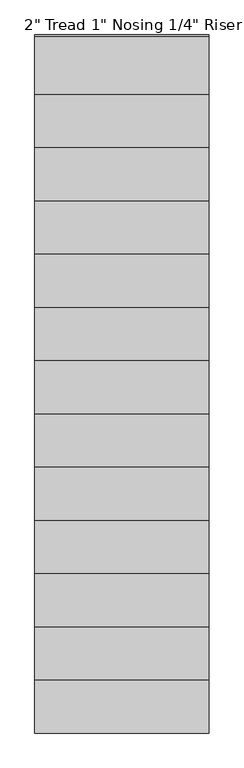
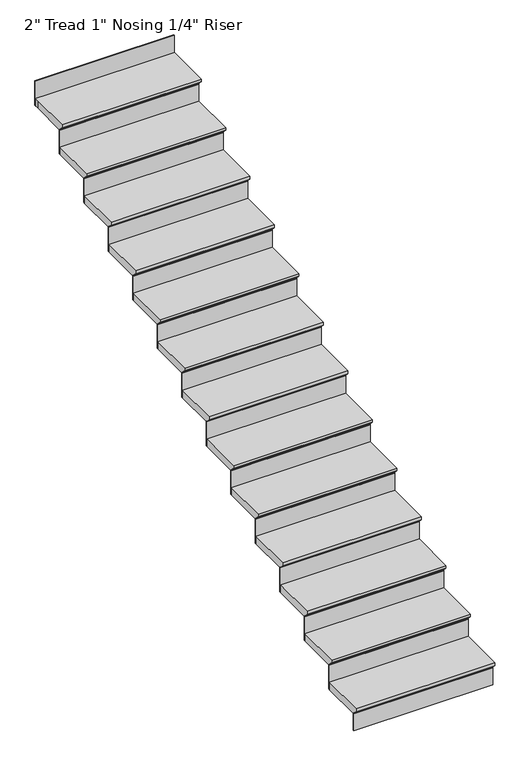
"""IFC4 building model written with IfcOpenShell, lengths in millimetres: stair flight geometry."""

from ifc_helpers import new_model, si_unit, origin, place, context, project, spatial, faceted_brep, source, transform, mapped, element, save


def stair_flight_ca28c9d9(model_context):
    return source(origin(), model_context, "Body", "Brep", [
        faceted_brep([(-2703.0415084, -23154.3851539, 34528.9005799), (-2703.0415084, -23154.3851539, 34547.9505799), (-3617.4415084, -23154.3851539, 34547.9505799), (-3617.4415084, -23154.3851539, 34528.9005799), (-2703.0415084, -23128.9851539, 34503.5005799), (-3617.4415084, -23128.9851539, 34503.5005799), (-2703.0415084, -22849.5851539, 34547.9505799), (-3617.4415084, -22849.5851539, 34547.9505799), (-3617.4415084, -23128.9851539, 34497.1505799), (-3617.4415084, -22849.5851539, 34497.1505799), (-2703.0415084, -22849.5851539, 34497.1505799), (-2703.0415084, -23128.9851539, 34497.1505799)], [[[0, 1, 2, 3]], [[4, 0, 3, 5]], [[2, 1, 6, 7]], [[8, 9, 10, 11]], [[2, 7, 9, 8, 5, 3]], [[8, 11, 4, 5]], [[6, 1, 0, 4, 11, 10]], [[7, 6, 10, 9]]]),
        faceted_brep([(-2703.0415084, -23128.9851539, 34497.1505799), (-2703.0415084, -23128.9851539, 34378.6172466), (-2703.0415084, -23122.6351539, 34378.6172466), (-2703.0415084, -23122.6351539, 34497.1505799), (-3617.4415084, -23128.9851539, 34497.1505799), (-3617.4415084, -23122.6351539, 34497.1505799), (-3617.4415084, -23122.6351539, 34378.6172466), (-3617.4415084, -23128.9851539, 34378.6172466)], [[[0, 1, 2, 3]], [[4, 5, 6, 7]], [[1, 0, 4, 7]], [[2, 1, 7, 6]], [[3, 2, 6, 5]], [[0, 3, 5, 4]]]),
        faceted_brep([(-2703.0415084, -22849.5851539, 34666.4839133), (-2703.0415084, -22849.5851539, 34497.1505799), (-2703.0415084, -22843.2351539, 34497.1505799), (-2703.0415084, -22843.2351539, 34666.4839133), (-3617.4415084, -22849.5851539, 34666.4839133), (-3617.4415084, -22843.2351539, 34666.4839133), (-3617.4415084, -22843.2351539, 34497.1505799), (-3617.4415084, -22849.5851539, 34497.1505799)], [[[0, 1, 2, 3]], [[4, 5, 6, 7]], [[1, 0, 4, 7]], [[2, 1, 7, 6]], [[3, 2, 6, 5]], [[0, 3, 5, 4]]]),
        faceted_brep([(-3617.4415084, -22874.9851539, 34717.2839133), (-2703.0415084, -22874.9851539, 34717.2839133), (-2703.0415084, -22570.1851539, 34717.2839133), (-3617.4415084, -22570.1851539, 34717.2839133), (-3617.4415084, -22849.5851539, 34666.4839133), (-3617.4415084, -22570.1851539, 34666.4839133), (-2703.0415084, -22570.1851539, 34666.4839133), (-2703.0415084, -22849.5851539, 34666.4839133), (-3617.4415084, -22849.5851539, 34672.8339133), (-3617.4415084, -22874.9851539, 34698.2339133), (-2703.0415084, -22849.5851539, 34672.8339133), (-2703.0415084, -22874.9851539, 34698.2339133)], [[[0, 1, 2, 3]], [[4, 5, 6, 7]], [[0, 3, 5, 4, 8, 9]], [[4, 7, 10, 8]], [[2, 1, 11, 10, 7, 6]], [[3, 2, 6, 5]], [[11, 1, 0, 9]], [[10, 11, 9, 8]]]),
        faceted_brep([(-2703.0415084, -22570.1851539, 34835.8172466), (-2703.0415084, -22570.1851539, 34666.4839133), (-2703.0415084, -22563.8351539, 34666.4839133), (-2703.0415084, -22563.8351539, 34835.8172466), (-3617.4415084, -22570.1851539, 34835.8172466), (-3617.4415084, -22563.8351539, 34835.8172466), (-3617.4415084, -22563.8351539, 34666.4839133), (-3617.4415084, -22570.1851539, 34666.4839133)], [[[0, 1, 2, 3]], [[4, 5, 6, 7]], [[1, 0, 4, 7]], [[2, 1, 7, 6]], [[3, 2, 6, 5]], [[0, 3, 5, 4]]]),
        faceted_brep([(-3617.4415084, -22595.5851539, 34886.6172466), (-2703.0415084, -22595.5851539, 34886.6172466), (-2703.0415084, -22290.7851539, 34886.6172466), (-3617.4415084, -22290.7851539, 34886.6172466), (-3617.4415084, -22570.1851539, 34835.8172466), (-3617.4415084, -22290.7851539, 34835.8172466), (-2703.0415084, -22290.7851539, 34835.8172466), (-2703.0415084, -22570.1851539, 34835.8172466), (-3617.4415084, -22570.1851539, 34842.1672466), (-3617.4415084, -22595.5851539, 34867.5672466), (-2703.0415084, -22570.1851539, 34842.1672466), (-2703.0415084, -22595.5851539, 34867.5672466)], [[[0, 1, 2, 3]], [[4, 5, 6, 7]], [[0, 3, 5, 4, 8, 9]], [[4, 7, 10, 8]], [[2, 1, 11, 10, 7, 6]], [[3, 2, 6, 5]], [[11, 1, 0, 9]], [[10, 11, 9, 8]]]),
        faceted_brep([(-2703.0415084, -22290.7851539, 35005.1505799), (-2703.0415084, -22290.7851539, 34835.8172466), (-2703.0415084, -22284.4351539, 34835.8172466), (-2703.0415084, -22284.4351539, 35005.1505799), (-3617.4415084, -22290.7851539, 35005.1505799), (-3617.4415084, -22284.4351539, 35005.1505799), (-3617.4415084, -22284.4351539, 34835.8172466), (-3617.4415084, -22290.7851539, 34835.8172466)], [[[0, 1, 2, 3]], [[4, 5, 6, 7]], [[1, 0, 4, 7]], [[2, 1, 7, 6]], [[3, 2, 6, 5]], [[0, 3, 5, 4]]]),
        faceted_brep([(-3617.4415084, -22316.1851539, 35055.9505799), (-2703.0415084, -22316.1851539, 35055.9505799), (-2703.0415084, -22011.3851539, 35055.9505799), (-3617.4415084, -22011.3851539, 35055.9505799), (-3617.4415084, -22290.7851539, 35005.1505799), (-3617.4415084, -22011.3851539, 35005.1505799), (-2703.0415084, -22011.3851539, 35005.1505799), (-2703.0415084, -22290.7851539, 35005.1505799), (-3617.4415084, -22290.7851539, 35011.5005799), (-3617.4415084, -22316.1851539, 35036.9005799), (-2703.0415084, -22290.7851539, 35011.5005799), (-2703.0415084, -22316.1851539, 35036.9005799)], [[[0, 1, 2, 3]], [[4, 5, 6, 7]], [[0, 3, 5, 4, 8, 9]], [[4, 7, 10, 8]], [[2, 1, 11, 10, 7, 6]], [[3, 2, 6, 5]], [[11, 1, 0, 9]], [[10, 11, 9, 8]]]),
        faceted_brep([(-2703.0415084, -22011.3851539, 35174.4839133), (-2703.0415084, -22011.3851539, 35005.1505799), (-2703.0415084, -22005.0351539, 35005.1505799), (-2703.0415084, -22005.0351539, 35174.4839133), (-3617.4415084, -22011.3851539, 35174.4839133), (-3617.4415084, -22005.0351539, 35174.4839133), (-3617.4415084, -22005.0351539, 35005.1505799), (-3617.4415084, -22011.3851539, 35005.1505799)], [[[0, 1, 2, 3]], [[4, 5, 6, 7]], [[1, 0, 4, 7]], [[2, 1, 7, 6]], [[3, 2, 6, 5]], [[0, 3, 5, 4]]]),
        faceted_brep([(-3617.4415084, -22036.7851539, 35225.2839133), (-2703.0415084, -22036.7851539, 35225.2839133), (-2703.0415084, -21731.9851539, 35225.2839133), (-3617.4415084, -21731.9851539, 35225.2839133), (-3617.4415084, -22011.3851539, 35174.4839133), (-3617.4415084, -21731.9851539, 35174.4839133), (-2703.0415084, -21731.9851539, 35174.4839133), (-2703.0415084, -22011.3851539, 35174.4839133), (-3617.4415084, -22011.3851539, 35180.8339133), (-3617.4415084, -22036.7851539, 35206.2339133), (-2703.0415084, -22011.3851539, 35180.8339133), (-2703.0415084, -22036.7851539, 35206.2339133)], [[[0, 1, 2, 3]], [[4, 5, 6, 7]], [[0, 3, 5, 4, 8, 9]], [[4, 7, 10, 8]], [[2, 1, 11, 10, 7, 6]], [[3, 2, 6, 5]], [[11, 1, 0, 9]], [[10, 11, 9, 8]]]),
        faceted_brep([(-2703.0415084, -21731.9851539, 35343.8172466), (-2703.0415084, -21731.9851539, 35174.4839133), (-2703.0415084, -21725.6351539, 35174.4839133), (-2703.0415084, -21725.6351539, 35343.8172466), (-3617.4415084, -21731.9851539, 35343.8172466), (-3617.4415084, -21725.6351539, 35343.8172466), (-3617.4415084, -21725.6351539, 35174.4839133), (-3617.4415084, -21731.9851539, 35174.4839133)], [[[0, 1, 2, 3]], [[4, 5, 6, 7]], [[1, 0, 4, 7]], [[2, 1, 7, 6]], [[3, 2, 6, 5]], [[0, 3, 5, 4]]]),
        faceted_brep([(-3617.4415084, -21757.3851539, 35394.6172466), (-2703.0415084, -21757.3851539, 35394.6172466), (-2703.0415084, -21452.5851539, 35394.6172466), (-3617.4415084, -21452.5851539, 35394.6172466), (-3617.4415084, -21731.9851539, 35343.8172466), (-3617.4415084, -21452.5851539, 35343.8172466), (-2703.0415084, -21452.5851539, 35343.8172466), (-2703.0415084, -21731.9851539, 35343.8172466), (-3617.4415084, -21731.9851539, 35350.1672466), (-3617.4415084, -21757.3851539, 35375.5672466), (-2703.0415084, -21731.9851539, 35350.1672466), (-2703.0415084, -21757.3851539, 35375.5672466)], [[[0, 1, 2, 3]], [[4, 5, 6, 7]], [[0, 3, 5, 4, 8, 9]], [[4, 7, 10, 8]], [[2, 1, 11, 10, 7, 6]], [[3, 2, 6, 5]], [[11, 1, 0, 9]], [[10, 11, 9, 8]]]),
        faceted_brep([(-2703.0415084, -21452.5851539, 35513.1505799), (-2703.0415084, -21452.5851539, 35343.8172466), (-2703.0415084, -21446.2351539, 35343.8172466), (-2703.0415084, -21446.2351539, 35513.1505799), (-3617.4415084, -21452.5851539, 35513.1505799), (-3617.4415084, -21446.2351539, 35513.1505799), (-3617.4415084, -21446.2351539, 35343.8172466), (-3617.4415084, -21452.5851539, 35343.8172466)], [[[0, 1, 2, 3]], [[4, 5, 6, 7]], [[1, 0, 4, 7]], [[2, 1, 7, 6]], [[3, 2, 6, 5]], [[0, 3, 5, 4]]]),
        faceted_brep([(-3617.4415084, -21477.9851539, 35563.9505799), (-2703.0415084, -21477.9851539, 35563.9505799), (-2703.0415084, -21173.1851539, 35563.9505799), (-3617.4415084, -21173.1851539, 35563.9505799), (-3617.4415084, -21452.5851539, 35513.1505799), (-3617.4415084, -21173.1851539, 35513.1505799), (-2703.0415084, -21173.1851539, 35513.1505799), (-2703.0415084, -21452.5851539, 35513.1505799), (-3617.4415084, -21452.5851539, 35519.5005799), (-3617.4415084, -21477.9851539, 35544.9005799), (-2703.0415084, -21452.5851539, 35519.5005799), (-2703.0415084, -21477.9851539, 35544.9005799)], [[[0, 1, 2, 3]], [[4, 5, 6, 7]], [[0, 3, 5, 4, 8, 9]], [[4, 7, 10, 8]], [[2, 1, 11, 10, 7, 6]], [[3, 2, 6, 5]], [[11, 1, 0, 9]], [[10, 11, 9, 8]]]),
        faceted_brep([(-2703.0415084, -21173.1851539, 35682.4839133), (-2703.0415084, -21173.1851539, 35513.1505799), (-2703.0415084, -21166.8351539, 35513.1505799), (-2703.0415084, -21166.8351539, 35682.4839133), (-3617.4415084, -21173.1851539, 35682.4839133), (-3617.4415084, -21166.8351539, 35682.4839133), (-3617.4415084, -21166.8351539, 35513.1505799), (-3617.4415084, -21173.1851539, 35513.1505799)], [[[0, 1, 2, 3]], [[4, 5, 6, 7]], [[1, 0, 4, 7]], [[2, 1, 7, 6]], [[3, 2, 6, 5]], [[0, 3, 5, 4]]]),
        faceted_brep([(-3617.4415084, -21198.5851539, 35733.2839133), (-2703.0415084, -21198.5851539, 35733.2839133), (-2703.0415084, -20893.7851539, 35733.2839133), (-3617.4415084, -20893.7851539, 35733.2839133), (-3617.4415084, -21173.1851539, 35682.4839133), (-3617.4415084, -20893.7851539, 35682.4839133), (-2703.0415084, -20893.7851539, 35682.4839133), (-2703.0415084, -21173.1851539, 35682.4839133), (-3617.4415084, -21173.1851539, 35688.8339133), (-3617.4415084, -21198.5851539, 35714.2339133), (-2703.0415084, -21173.1851539, 35688.8339133), (-2703.0415084, -21198.5851539, 35714.2339133)], [[[0, 1, 2, 3]], [[4, 5, 6, 7]], [[0, 3, 5, 4, 8, 9]], [[4, 7, 10, 8]], [[2, 1, 11, 10, 7, 6]], [[3, 2, 6, 5]], [[11, 1, 0, 9]], [[10, 11, 9, 8]]]),
        faceted_brep([(-2703.0415084, -20893.7851539, 35851.8172466), (-2703.0415084, -20893.7851539, 35682.4839133), (-2703.0415084, -20887.4351539, 35682.4839133), (-2703.0415084, -20887.4351539, 35851.8172466), (-3617.4415084, -20893.7851539, 35851.8172466), (-3617.4415084, -20887.4351539, 35851.8172466), (-3617.4415084, -20887.4351539, 35682.4839133), (-3617.4415084, -20893.7851539, 35682.4839133)], [[[0, 1, 2, 3]], [[4, 5, 6, 7]], [[1, 0, 4, 7]], [[2, 1, 7, 6]], [[3, 2, 6, 5]], [[0, 3, 5, 4]]]),
        faceted_brep([(-3617.4415084, -20919.1851539, 35902.6172466), (-2703.0415084, -20919.1851539, 35902.6172466), (-2703.0415084, -20614.3851539, 35902.6172466), (-3617.4415084, -20614.3851539, 35902.6172466), (-3617.4415084, -20893.7851539, 35851.8172466), (-3617.4415084, -20614.3851539, 35851.8172466), (-2703.0415084, -20614.3851539, 35851.8172466), (-2703.0415084, -20893.7851539, 35851.8172466), (-3617.4415084, -20893.7851539, 35858.1672466), (-3617.4415084, -20919.1851539, 35883.5672466), (-2703.0415084, -20893.7851539, 35858.1672466), (-2703.0415084, -20919.1851539, 35883.5672466)], [[[0, 1, 2, 3]], [[4, 5, 6, 7]], [[0, 3, 5, 4, 8, 9]], [[4, 7, 10, 8]], [[2, 1, 11, 10, 7, 6]], [[3, 2, 6, 5]], [[11, 1, 0, 9]], [[10, 11, 9, 8]]]),
        faceted_brep([(-2703.0415084, -20614.3851539, 36021.1505799), (-2703.0415084, -20614.3851539, 35851.8172466), (-2703.0415084, -20608.0351539, 35851.8172466), (-2703.0415084, -20608.0351539, 36021.1505799), (-3617.4415084, -20614.3851539, 36021.1505799), (-3617.4415084, -20608.0351539, 36021.1505799), (-3617.4415084, -20608.0351539, 35851.8172466), (-3617.4415084, -20614.3851539, 35851.8172466)], [[[0, 1, 2, 3]], [[4, 5, 6, 7]], [[1, 0, 4, 7]], [[2, 1, 7, 6]], [[3, 2, 6, 5]], [[0, 3, 5, 4]]]),
        faceted_brep([(-3617.4415084, -20639.7851539, 36071.9505799), (-2703.0415084, -20639.7851539, 36071.9505799), (-2703.0415084, -20334.9851539, 36071.9505799), (-3617.4415084, -20334.9851539, 36071.9505799), (-3617.4415084, -20614.3851539, 36021.1505799), (-3617.4415084, -20334.9851539, 36021.1505799), (-2703.0415084, -20334.9851539, 36021.1505799), (-2703.0415084, -20614.3851539, 36021.1505799), (-3617.4415084, -20614.3851539, 36027.5005799), (-3617.4415084, -20639.7851539, 36052.9005799), (-2703.0415084, -20614.3851539, 36027.5005799), (-2703.0415084, -20639.7851539, 36052.9005799)], [[[0, 1, 2, 3]], [[4, 5, 6, 7]], [[0, 3, 5, 4, 8, 9]], [[4, 7, 10, 8]], [[2, 1, 11, 10, 7, 6]], [[3, 2, 6, 5]], [[11, 1, 0, 9]], [[10, 11, 9, 8]]]),
        faceted_brep([(-2703.0415084, -20334.9851539, 36190.4839133), (-2703.0415084, -20334.9851539, 36021.1505799), (-2703.0415084, -20328.6351539, 36021.1505799), (-2703.0415084, -20328.6351539, 36190.4839133), (-3617.4415084, -20334.9851539, 36190.4839133), (-3617.4415084, -20328.6351539, 36190.4839133), (-3617.4415084, -20328.6351539, 36021.1505799), (-3617.4415084, -20334.9851539, 36021.1505799)], [[[0, 1, 2, 3]], [[4, 5, 6, 7]], [[1, 0, 4, 7]], [[2, 1, 7, 6]], [[3, 2, 6, 5]], [[0, 3, 5, 4]]]),
        faceted_brep([(-3617.4415084, -20360.3851539, 36241.2839133), (-2703.0415084, -20360.3851539, 36241.2839133), (-2703.0415084, -20055.5851539, 36241.2839133), (-3617.4415084, -20055.5851539, 36241.2839133), (-3617.4415084, -20334.9851539, 36190.4839133), (-3617.4415084, -20055.5851539, 36190.4839133), (-2703.0415084, -20055.5851539, 36190.4839133), (-2703.0415084, -20334.9851539, 36190.4839133), (-3617.4415084, -20334.9851539, 36196.8339133), (-3617.4415084, -20360.3851539, 36222.2339133), (-2703.0415084, -20334.9851539, 36196.8339133), (-2703.0415084, -20360.3851539, 36222.2339133)], [[[0, 1, 2, 3]], [[4, 5, 6, 7]], [[0, 3, 5, 4, 8, 9]], [[4, 7, 10, 8]], [[2, 1, 11, 10, 7, 6]], [[3, 2, 6, 5]], [[11, 1, 0, 9]], [[10, 11, 9, 8]]]),
        faceted_brep([(-2703.0415084, -20055.5851539, 36359.8172466), (-2703.0415084, -20055.5851539, 36190.4839133), (-2703.0415084, -20049.2351539, 36190.4839133), (-2703.0415084, -20049.2351539, 36359.8172466), (-3617.4415084, -20055.5851539, 36359.8172466), (-3617.4415084, -20049.2351539, 36359.8172466), (-3617.4415084, -20049.2351539, 36190.4839133), (-3617.4415084, -20055.5851539, 36190.4839133)], [[[0, 1, 2, 3]], [[4, 5, 6, 7]], [[1, 0, 4, 7]], [[2, 1, 7, 6]], [[3, 2, 6, 5]], [[0, 3, 5, 4]]]),
        faceted_brep([(-3617.4415084, -20080.9851539, 36410.6172466), (-2703.0415084, -20080.9851539, 36410.6172466), (-2703.0415084, -19776.1851539, 36410.6172466), (-3617.4415084, -19776.1851539, 36410.6172466), (-3617.4415084, -20055.5851539, 36359.8172466), (-3617.4415084, -19776.1851539, 36359.8172466), (-2703.0415084, -19776.1851539, 36359.8172466), (-2703.0415084, -20055.5851539, 36359.8172466), (-3617.4415084, -20055.5851539, 36366.1672466), (-3617.4415084, -20080.9851539, 36391.5672466), (-2703.0415084, -20055.5851539, 36366.1672466), (-2703.0415084, -20080.9851539, 36391.5672466)], [[[0, 1, 2, 3]], [[4, 5, 6, 7]], [[0, 3, 5, 4, 8, 9]], [[4, 7, 10, 8]], [[2, 1, 11, 10, 7, 6]], [[3, 2, 6, 5]], [[11, 1, 0, 9]], [[10, 11, 9, 8]]]),
        faceted_brep([(-2703.0415084, -19496.7851539, 36698.4839133), (-2703.0415084, -19496.7851539, 36529.1505799), (-2703.0415084, -19490.4351539, 36529.1505799), (-2703.0415084, -19490.4351539, 36698.4839133), (-3617.4415084, -19496.7851539, 36698.4839133), (-3617.4415084, -19490.4351539, 36698.4839133), (-3617.4415084, -19490.4351539, 36529.1505799), (-3617.4415084, -19496.7851539, 36529.1505799)], [[[0, 1, 2, 3]], [[4, 5, 6, 7]], [[1, 0, 4, 7]], [[2, 1, 7, 6]], [[3, 2, 6, 5]], [[0, 3, 5, 4]]]),
        faceted_brep([(-2703.0415084, -19776.1851539, 36529.1505799), (-2703.0415084, -19776.1851539, 36359.8172466), (-2703.0415084, -19769.8351539, 36359.8172466), (-2703.0415084, -19769.8351539, 36529.1505799), (-3617.4415084, -19776.1851539, 36529.1505799), (-3617.4415084, -19769.8351539, 36529.1505799), (-3617.4415084, -19769.8351539, 36359.8172466), (-3617.4415084, -19776.1851539, 36359.8172466)], [[[0, 1, 2, 3]], [[4, 5, 6, 7]], [[1, 0, 4, 7]], [[2, 1, 7, 6]], [[3, 2, 6, 5]], [[0, 3, 5, 4]]]),
        faceted_brep([(-3617.4415084, -19496.7851539, 36579.9505799), (-3617.4415084, -19522.1851539, 36579.9505799), (-3617.4415084, -19801.5851539, 36579.9505799), (-2703.0415084, -19801.5851539, 36579.9505799), (-2703.0415084, -19496.7851539, 36579.9505799), (-3617.4415084, -19522.1851539, 36529.1505799), (-3617.4415084, -19496.7851539, 36529.1505799), (-2703.0415084, -19496.7851539, 36529.1505799), (-2703.0415084, -19776.1851539, 36529.1505799), (-3617.4415084, -19776.1851539, 36529.1505799), (-3617.4415084, -19776.1851539, 36535.5005799), (-3617.4415084, -19801.5851539, 36560.9005799), (-2703.0415084, -19776.1851539, 36535.5005799), (-2703.0415084, -19801.5851539, 36560.9005799)], [[[0, 1, 2, 3, 4]], [[5, 6, 7, 8, 9]], [[1, 0, 6, 5]], [[2, 1, 5, 9, 10, 11]], [[9, 8, 12, 10]], [[4, 3, 13, 12, 8, 7]], [[0, 4, 7, 6]], [[13, 3, 2, 11]], [[12, 13, 11, 10]]]),
    ])


if __name__ == "__main__":
    model = new_model("IFC4")
    model_context = context("Model", 3, world=origin())
    ifc_project = project(units=[si_unit("LENGTHUNIT", "METRE", prefix="MILLI")], contexts=[model_context])
    site = spatial("IfcSite", under=ifc_project)
    building = spatial("IfcBuilding", under=site)
    placement = place(None, origin())
    stair_flight_shape = stair_flight_ca28c9d9(model_context)
    element("IfcStairFlight", 1, ObjectType="2\" Tread 1\" Nosing 1/4\" Riser", at=placement, inside=building, context=model_context, shape_type="MappedRepresentation", body=[
        mapped(stair_flight_shape, transform((0.0, 0.0, 0.0), x_axis=(1.0, 0.0, 0.0), y_axis=(0.0, 1.0, 0.0), z_axis=(0.0, 0.0, 1.0))),
    ])
    save(model, "model.ifc")
